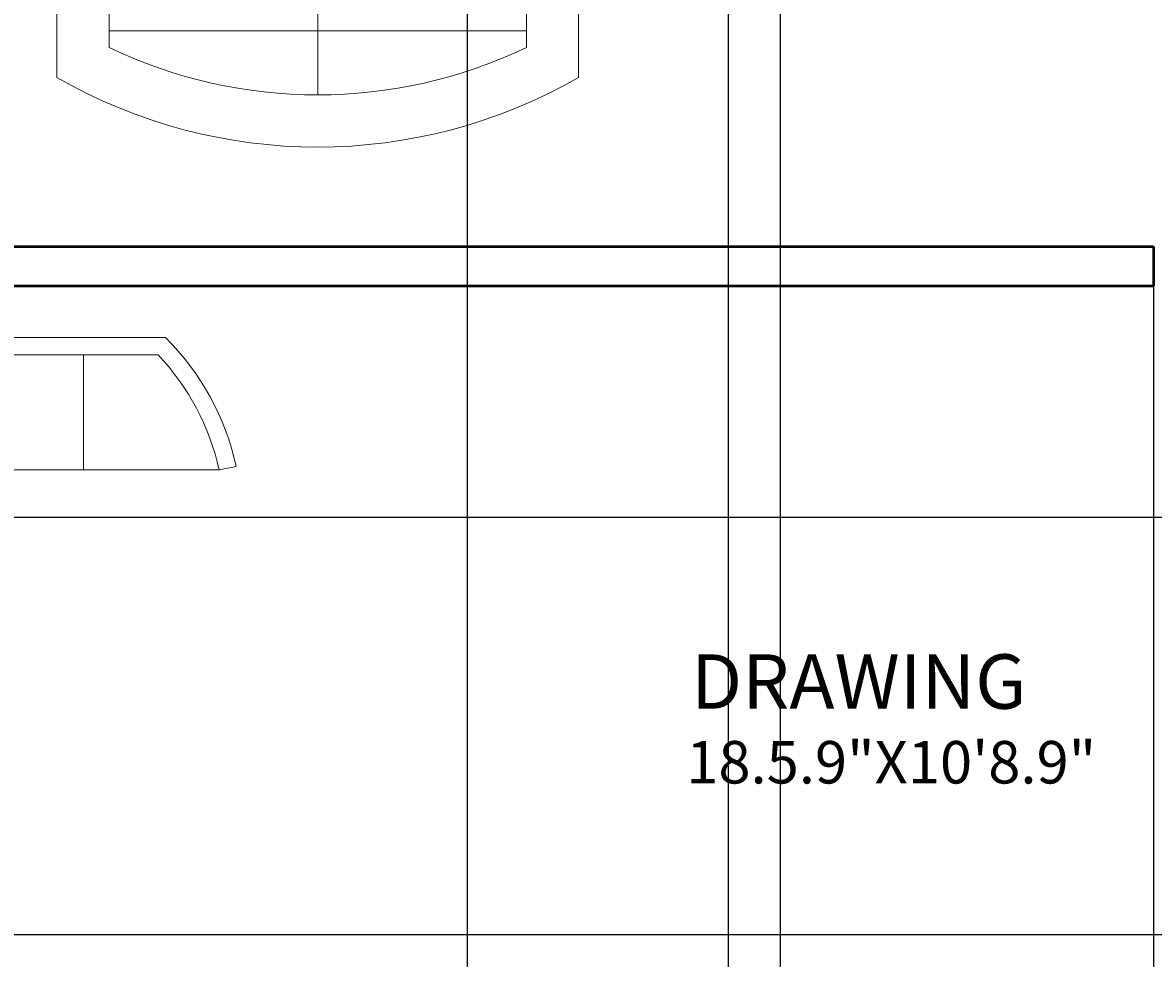
# Model space of a CAD drawing. Units: inches. Extents: x 7359 to 7979, y 33027 to 34263.
# Tile 26 of 32: x 7511 to 7641, y 33825 to 33933. Entities that reach past the tile are written whole.
import ezdxf

# ---------------------------------------------------------------- set-up
doc = ezdxf.new("R2010")
doc.units = ezdxf.units.IN
for name, color, linetype, lineweight in [('A-ANNO-DIMS', 2, 'Continuous', 18), ('A-AREA-IDEN', 7, 'Continuous', 18), ('A-FURN', 8, 'Continuous', 18), ('A-WALL', 7, 'Continuous', 50)]:
    doc.layers.add(name, color=color, linetype=linetype, lineweight=lineweight)
doc.styles.get("Standard").update_dxf_attribs({"font": 'arial.ttf'})
doc.dimstyles.get("Standard").update_dxf_attribs({"dimtxt": 0.18, "dimasz": 0.18, "dimexe": 0.18, "dimexo": 0.0625, "dimgap": 0.09, "dimtad": 0, "dimtih": 1, "dimtoh": 1, "dimdec": 4, "dimzin": 0, "dimdsep": 46, "dimtxsty": 'Standard', "dimcen": 0.09, "dimadec": 0, "dimazin": 0, "dimtfac": 1, "dimtdec": 4, "dimtofl": 0, "dimtmove": 0, "dimatfit": 3, "dimfxl": 1, "dimtolj": 1, "dimtzin": 0, "dimarcsym": 0})

# ---------------------------------------------------------------- blocks, each defined once
blk = doc.blocks.new('Sofa - Roundback Loveseat 5 ft.')
for p, q in [((0, -32.44198), (0, -5.99998)), ((-24, -33.99998), (-24, -11.46958)), ((24.00004, -33.99998), (24.00004, -11.46958)), ((-23.9998, -13.38178), (23.99986, -13.38178)), ((-24, -32.44198), (24.00004, -32.44198))]:
    blk.add_line(p, q)
for points in [[(-24, -33.99998), (-30, -33.99998), (-30, -7.99998)], [(30.00004, -7.99998), (30.00004, -33.99998), (24.00004, -33.99998)]]:
    blk.add_lwpolyline(points)
for centre, radius, start, end in [((0, -60.24998), 60.24998, 60.13715, 119.8628), ((0, -61.38438), 55.38444, 64.32083, 115.6792)]:
    blk.add_arc(centre, radius, start, end)
blk = doc.blocks.new('SOFA-CORNER')
for p, q in [((19.3, 69.98), (52.27, 69.98)), ((19.51, 67.98), (51.43, 67.98)), ((27.06, 54.75), (27.06, 67.98)), ((42.86, 54.75), (42.86, 67.98)), ((22.35, 54.75), (58.44, 54.75)), ((58.44, 54.75), (60.39, 55.17)), ((0, 8.53), (0, 48.06)), ((2, 9.3), (2, 48.06)), ((15.59, 46.88), (2, 46.88)), ((15.16, 44.58), (15.16, 1.96)), ((15.16, 33.02), (2, 33.02)), ((15.16, 18.66), (2, 18.66)), ((14.78, 0), (15.16, 1.96))]:
    blk.add_line(p, q)
for centre, radius, start, end in [((24.48, 45.95), 24.58, 102.1798, 174.6548), ((31.37, 48.88), 29.7, 12.2304, 45.2702), ((24.48, 45.95), 22.58, 102.7099, 174.6548), ((31.37, 48.88), 27.7, 12.2304, 43.5923), ((27.51, 43.47), 12.4, 114.5692, 174.8439), ((19.72, 25.63), 24.1, 222.6619, 259.0828), ((19.72, 25.63), 26.1, 220.9183, 259.0828)]:
    blk.add_arc(centre, radius, start, end)
blk = doc.blocks.new('*D68')
at = {"layer": 'A-ANNO-DIMS', "color": 0, "lineweight": -2, "transparency": 16777216}
for p, q in [((7562.59, 34181.77), (7562.59, 33632.31)), ((7592.59, 34181.77), (7592.59, 33632.31)), ((7562.77, 33632.49), (7577.37, 33632.49)), ((7592.41, 33632.49), (7577.81, 33632.49))]:
    blk.add_line(p, q, dxfattribs=at)
at = {"layer": 'A-ANNO-DIMS', "color": 0, "transparency": 16777216}
for points in [[(7562.77, 33632.52), (7562.77, 33632.46), (7562.59, 33632.49)], [(7592.41, 33632.52), (7592.41, 33632.46), (7592.59, 33632.49)]]:
    blk.add_solid(points, dxfattribs=at)
at = {"layer": 'Defpoints', "color": 0, "transparency": 16777216}
for p in [(7562.59, 34181.83), (7592.59, 34181.83), (7592.59, 33632.49)]:
    blk.add_point(p, dxfattribs=at)
at = {"layer": 'A-ANNO-DIMS', "color": 0, "transparency": 16777216, "insert": (7577.59, 33632.49), "char_height": 0.18, "attachment_point": 5}
blk.add_mtext('\\A1;30', dxfattribs=at)
blk = doc.blocks.new('*D71')
at = {"layer": 'A-ANNO-DIMS', "color": 0, "lineweight": -2, "transparency": 16777216}
for p, q in [((7641.49, 33907.17), (7641.49, 33632.31)), ((7683.49, 33907.17), (7683.49, 33632.31)), ((7641.67, 33632.49), (7662.27, 33632.49)), ((7683.31, 33632.49), (7662.71, 33632.49))]:
    blk.add_line(p, q, dxfattribs=at)
at = {"layer": 'A-ANNO-DIMS', "color": 0, "transparency": 16777216}
for points in [[(7641.67, 33632.52), (7641.67, 33632.46), (7641.49, 33632.49)], [(7683.31, 33632.52), (7683.31, 33632.46), (7683.49, 33632.49)]]:
    blk.add_solid(points, dxfattribs=at)
at = {"layer": 'Defpoints', "color": 0, "transparency": 16777216}
for p in [(7641.49, 33907.23), (7683.49, 33907.23), (7683.49, 33632.49)]:
    blk.add_point(p, dxfattribs=at)
at = {"layer": 'A-ANNO-DIMS', "color": 0, "transparency": 16777216, "insert": (7662.49, 33632.49), "char_height": 0.18, "attachment_point": 5}
blk.add_mtext('\\A1;42', dxfattribs=at)
blk = doc.blocks.new('*D72')
at = {"layer": 'A-ANNO-DIMS', "color": 0, "lineweight": -2, "transparency": 16777216}
for p, q in [((7689.43, 33876.08), (7359.41, 33876.08)), ((7359.59, 33875.9), (7359.59, 33852.27)), ((7359.59, 33828.26), (7359.59, 33851.9)), ((7689.43, 33828.08), (7359.41, 33828.08))]:
    blk.add_line(p, q, dxfattribs=at)
at = {"layer": 'A-ANNO-DIMS', "color": 0, "transparency": 16777216}
for points in [[(7359.56, 33875.9), (7359.62, 33875.9), (7359.59, 33876.08)], [(7359.56, 33828.26), (7359.62, 33828.26), (7359.59, 33828.08)]]:
    blk.add_solid(points, dxfattribs=at)
at = {"layer": 'Defpoints', "color": 0, "transparency": 16777216}
for p in [(7359.59, 33876.08), (7689.49, 33876.08), (7689.49, 33828.08)]:
    blk.add_point(p, dxfattribs=at)
at = {"layer": 'A-ANNO-DIMS', "color": 0, "transparency": 16777216, "insert": (7359.59, 33852.08), "char_height": 0.18, "attachment_point": 5}
blk.add_mtext('\\A1;48', dxfattribs=at)
blk = doc.blocks.new('*D83')
at = {"layer": 'A-ANNO-DIMS', "color": 0, "lineweight": -2, "transparency": 16777216}
for p, q in [((7592.591484, 34081.771428), (7592.591484, 33632.309146)), ((7598.591484, 34081.771428), (7598.591484, 33632.309146)), ((7592.771484, 33632.489146), (7595.442057, 33632.489146)), ((7598.411484, 33632.489146), (7595.740911, 33632.489146))]:
    blk.add_line(p, q, dxfattribs=at)
at = {"layer": 'A-ANNO-DIMS', "color": 0, "transparency": 16777216}
for points in [[(7592.771484, 33632.519146), (7592.771484, 33632.459146), (7592.591484, 33632.489146)], [(7598.411484, 33632.519146), (7598.411484, 33632.459146), (7598.591484, 33632.489146)]]:
    blk.add_solid(points, dxfattribs=at)
at = {"layer": 'Defpoints', "color": 0, "transparency": 16777216}
for p in [(7592.591484, 34081.833928), (7598.591484, 34081.833928), (7598.591484, 33632.489146)]:
    blk.add_point(p, dxfattribs=at)
at = {"layer": 'A-ANNO-DIMS', "color": 0, "transparency": 16777216, "insert": (7595.591484, 33632.489146), "char_height": 0.18, "attachment_point": 5}
blk.add_mtext('\\A1;6', dxfattribs=at)

msp = doc.modelspace()

# ---------------------------------------------------------------- linework, layer by layer
at = {"layer": 'A-WALL'}
for p, q in [((7467.5915, 33907.2339), (7641.4915, 33907.2339)), ((7641.4915, 33907.2339), (7641.4915, 33902.7339)), ((7467.5915, 33902.7339), (7641.4915, 33902.7339))]:
    msp.add_line(p, q, dxfattribs=at)

# ---------------------------------------------------------------- block references
at = {"layer": 'A-FURN', "xscale": -1, "rotation": 180}
msp.add_blockref('Sofa - Roundback Loveseat 5 ft.', (7545.3969, 33918.6792), dxfattribs=at)
at = {"layer": 'A-FURN'}
msp.add_blockref('SOFA-CORNER', (7475.615, 33826.797), dxfattribs=at)

# ---------------------------------------------------------------- texts
at = {"layer": 'A-AREA-IDEN'}
for s, height, p in [('DRAWING', 6.25941, (7588.3341, 33854.0903)), ('18.5.9"X10\'8.9"', 4.885549, (7587.7709, 33845.4959))]:
    msp.add_text(s, height=height, dxfattribs=at).set_placement(p)

# ---------------------------------------------------------------- dimensions: what is measured, and where the dimension line sits
at = {"layer": 'A-ANNO-DIMS'}
for base, p1, p2, picture, middle in [((7592.5915, 33632.4891), (7562.5915, 34181.8339), (7592.5915, 34181.8339), '*D68', (7577.5915, 33632.4891)), ((7598.5915, 33632.4891), (7592.5915, 34081.8339), (7598.5915, 34081.8339), '*D83', (7595.5915, 33632.4891)), ((7683.4915, 33632.4891), (7641.4915, 33907.2339), (7683.4915, 33907.2339), '*D71', (7662.4915, 33632.4891))]:
    dim = msp.add_linear_dim(base=base, p1=p1, p2=p2, dimstyle='Standard', override={"dimdec": 0, "dimlfac": 1, "dimrnd": 0, "dimzin": 0, "dimdsep": 46, "dimlunit": 2}, dxfattribs=at)
    dim.commit()
    dim.dimension.update_dxf_attribs({"geometry": picture, "text_midpoint": middle})
dim = msp.add_linear_dim(base=(7359.5866, 33876.0839), p1=(7689.4915, 33828.0839), p2=(7689.4915, 33876.0839), angle=90, dimstyle='Standard', override={"dimdec": 0, "dimlfac": 1, "dimrnd": 0, "dimzin": 0, "dimdsep": 46, "dimlunit": 2}, dxfattribs=at)
dim.commit()
dim.dimension.update_dxf_attribs({"geometry": '*D72', "text_midpoint": (7359.5866, 33852.0839)})

doc.saveas('drawing.dxf')
